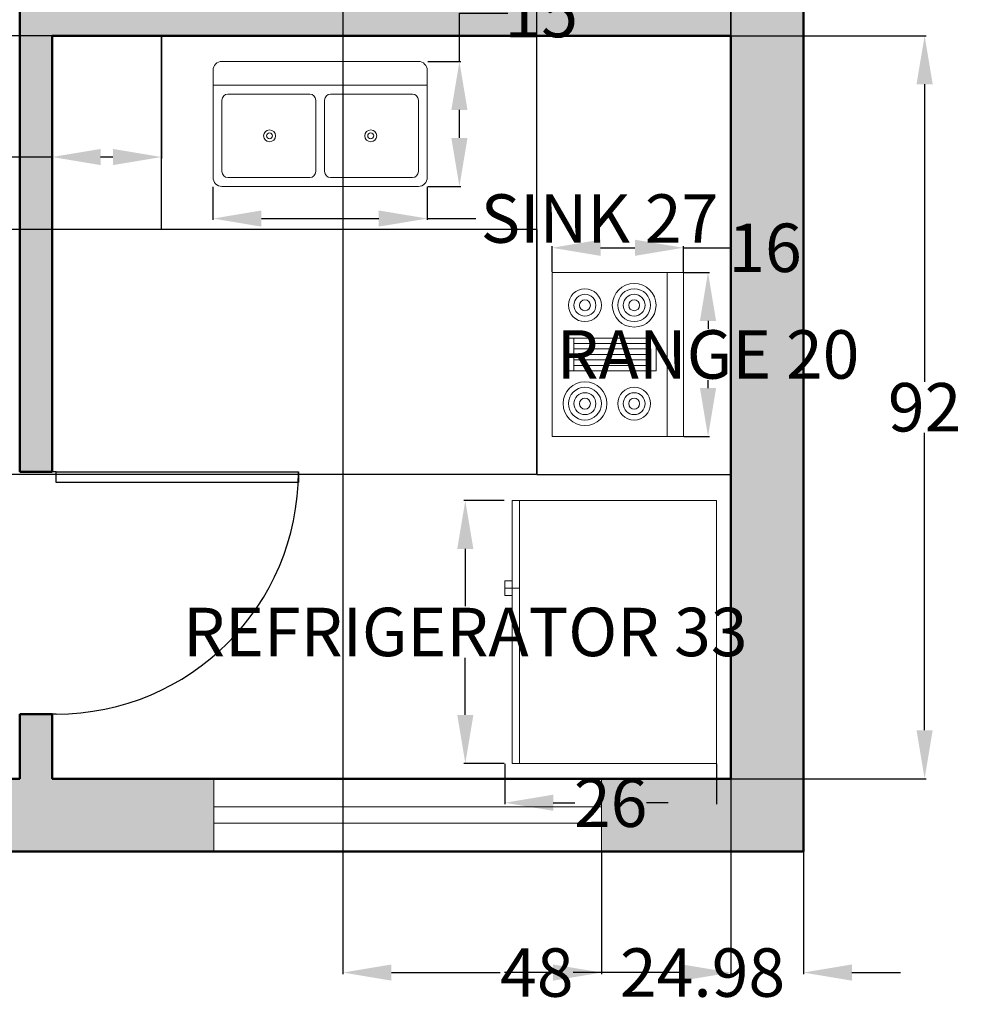
# Model space of a CAD drawing. Units: inches. Extents: x -11 to 341, y -300 to 41.
# Tile 4 of 5: x 192 to 308, y -300 to -178. Entities that reach past the tile are written whole.
import ezdxf

# ---------------------------------------------------------------- set-up
doc = ezdxf.new("R2010")
doc.units = ezdxf.units.IN
doc.header["$MEASUREMENT"] = 0
for name, color, linetype, lineweight in [('A-ANNO-DIMS', 2, 'Continuous', 18), ('A-DOOR', 3, 'Continuous', 25), ('A-EQPM', 8, 'Continuous', 18), ('A-FLOR-CASE', 8, 'Continuous', 25), ('A-FLOR-FIXT', 9, 'Continuous', 18), ('A-GLAZ', 4, 'Continuous', 18), ('A-WALL', 7, 'Continuous', 50), ('A-WALL-PATT', 251, 'Continuous', 13)]:
    doc.layers.add(name, color=color, linetype=linetype, lineweight=lineweight)
doc.styles.get("Standard").update_dxf_attribs({"font": 'arial.ttf'})
doc.dimstyles.get("Standard").update_dxf_attribs({"dimtxt": 6, "dimasz": 6, "dimexe": 0.18, "dimexo": 0.0625, "dimgap": 0.09, "dimtad": 0, "dimtih": 1, "dimtoh": 1, "dimdec": 0, "dimzin": 0, "dimdsep": 46, "dimlunit": 4, "dimtxsty": 'Standard', "dimcen": 0.09, "dimadec": 0, "dimazin": 0, "dimtfac": 1, "dimtdec": 0, "dimtofl": 0, "dimtmove": 0, "dimatfit": 3, "dimfxl": 1, "dimtolj": 1, "dimtzin": 0, "dimarcsym": 0})

# ---------------------------------------------------------------- blocks, each defined once
blk = doc.blocks.new('*U12')
for p, q in [((0, 0), (0, -6)), ((40, 0), (40, -6))]:
    blk.add_line(p, q)
blk.add_lwpolyline([(0, 0), (0, 40), (1.75, 40), (1.75, 0)], close=True)
blk.add_arc((0, 0), 40, 0, 90)
blk = doc.blocks.new('Range-Oven - 30 in top')
for p, q in [((0, -3), (30, -3)), ((12, -6), (18, -6)), ((13, -20), (13, -6)), ((14, -6), (14, -20)), ((15, -20), (15, -6)), ((16, -6), (16, -20)), ((17, -20), (17, -6)), ((18, -20), (12, -20))]:
    blk.add_line(p, q)
for points in [[(0, -24), (0, 0), (30, 0), (30, -24)], [(12, -21), (12, -5), (18, -5), (18, -21)]]:
    blk.add_lwpolyline(points, close=True)
for centre, radius in [((6, -9), 4), ((6, -9), 3), ((6, -9), 2), ((24, -9), 3), ((24, -9), 2), ((6, -9), 1), ((24, -9), 1), ((24, -18), 4), ((6, -18), 3), ((6, -18), 2), ((24, -18), 3), ((24, -18), 2), ((6, -18), 1), ((24, -18), 1)]:
    blk.add_circle(centre, radius)
blk = doc.blocks.new('Sink-double - 36 in top')
for p, q in [((-18, -4), (18, -4)), ((-0.75, -18.5), (-0.75, -6.5)), ((0.75, -6.5), (0.75, -18.5))]:
    blk.add_line(p, q)
for points in [[(-16.5, 0), (16.5, 0)], [(-18, -19.5), (-18, -1.5)], [(18, -1.5), (18, -19.5)], [(-16.5, -18.5), (-16.5, -6.5)], [(-15.5, -5.5), (-1.75, -5.5)], [(1.75, -5.5), (15.5, -5.5)], [(16.5, -6.5), (16.5, -18.5)], [(-1.75, -19.5), (-15.5, -19.5)], [(15.5, -19.5), (1.75, -19.5)], [(16.5, -21), (-16.5, -21)]]:
    blk.add_lwpolyline(points)
for centre, radius in [((-8.5, -12.5), 1), ((8.5, -12.5), 1), ((-8.5, -12.5), 0.5), ((8.5, -12.5), 0.5)]:
    blk.add_circle(centre, radius)
for centre, radius, start, end in [((-16.5, -1.5), 1.5, 90, 180), ((16.5, -1.5), 1.5, 0, 90), ((-15.5, -6.5), 1, 90, 180), ((-1.75, -6.5), 1, 0, 90), ((1.75, -6.5), 1, 90, 180), ((15.5, -6.5), 1, 0, 90), ((-16.5, -19.5), 1.5, 180, 270), ((-15.5, -18.5), 1, 180, 270), ((-1.75, -18.5), 1, 270, 0), ((1.75, -18.5), 1, 180, 270), ((15.5, -18.5), 1, 270, 0), ((16.5, -19.5), 1.5, 270, 0)]:
    blk.add_arc(centre, radius, start, end)
blk = doc.blocks.new('Refrigerator-2 door - 36 in top')
for p, q in [((0, -26.999999), (36, -26.999999)), ((11, -27.999999), (11, -28.999999)), ((12, -26.999999), (12, -28.999999)), ((13, -28.999999), (13, -27.999999)), ((11, -28.999999), (13, -28.999999))]:
    blk.add_line(p, q)
blk.add_lwpolyline([(0, -27.999999), (0, 0), (36, 0), (36, -27.999999)], close=True)
blk = doc.blocks.new('WIN-48IN')
for p, q in [((0, 0), (0, 9)), ((48, 9), (48, 0)), ((0, 5.5), (48, 5.5)), ((0, 3.5), (48, 3.5))]:
    blk.add_line(p, q)
blk = doc.blocks.new('*D35')
at = {"layer": 'A-ANNO-DIMS', "color": 0, "lineweight": -2, "transparency": 16777216}
for p, q in [((273.78, -208.9), (276.94, -208.9)), ((276.76, -214.9), (276.76, -215.87)), ((276.76, -223.22), (276.76, -222.25)), ((273.78, -229.22), (276.94, -229.22))]:
    blk.add_line(p, q, dxfattribs=at)
at = {"layer": 'A-ANNO-DIMS', "color": 0, "transparency": 16777216}
for points in [[(275.76, -214.9), (277.76, -214.9), (276.76, -208.9)], [(275.76, -223.22), (277.76, -223.22), (276.76, -229.22)]]:
    blk.add_solid(points, dxfattribs=at)
at = {"layer": 'Defpoints', "color": 0, "transparency": 16777216}
for p in [(273.72, -208.9), (273.72, -229.22), (276.76, -229.22)]:
    blk.add_point(p, dxfattribs=at)
at = {"layer": 'A-ANNO-DIMS', "color": 0, "transparency": 16777216, "insert": (276.76, -219.06), "char_height": 6, "attachment_point": 5}
blk.add_mtext('\\A1;RANGE 20', dxfattribs=at)
blk = doc.blocks.new('*D36')
at = {"layer": 'A-ANNO-DIMS', "color": 0, "lineweight": -2, "transparency": 16777216}
for p, q in [((257.46, -208.84), (257.46, -205.67)), ((263.46, -205.85), (267.72, -205.85)), ((273.72, -208.84), (273.72, -205.67)), ((273.72, -205.85), (279.72, -205.85))]:
    blk.add_line(p, q, dxfattribs=at)
at = {"layer": 'A-ANNO-DIMS', "color": 0, "transparency": 16777216}
for points in [[(263.46, -204.85), (263.46, -206.85), (257.46, -205.85)], [(267.72, -204.85), (267.72, -206.85), (273.72, -205.85)]]:
    blk.add_solid(points, dxfattribs=at)
at = {"layer": 'Defpoints', "color": 0, "transparency": 16777216}
for p in [(273.72, -205.85), (257.46, -208.9), (273.72, -208.9)]:
    blk.add_point(p, dxfattribs=at)
at = {"layer": 'A-ANNO-DIMS', "color": 0, "transparency": 16777216, "insert": (283.82, -205.85), "char_height": 6, "attachment_point": 5}
blk.add_mtext('\\A1;16', dxfattribs=at)
blk = doc.blocks.new('*D37')
at = {"layer": 'A-ANNO-DIMS', "color": 0, "lineweight": -2, "transparency": 16777216}
for p, q in [((215.49, -198.31), (215.49, -202.41)), ((242.01, -198.31), (242.01, -202.41)), ((221.49, -202.23), (236.01, -202.23)), ((242.01, -202.23), (248.01, -202.23))]:
    blk.add_line(p, q, dxfattribs=at)
at = {"layer": 'A-ANNO-DIMS', "color": 0, "transparency": 16777216}
for points in [[(221.49, -201.23), (221.49, -203.23), (215.49, -202.23)], [(236.01, -201.23), (236.01, -203.23), (242.01, -202.23)]]:
    blk.add_solid(points, dxfattribs=at)
at = {"layer": 'Defpoints', "color": 0, "transparency": 16777216}
for p in [(215.49, -198.25), (242.01, -198.25), (242.01, -202.23)]:
    blk.add_point(p, dxfattribs=at)
at = {"layer": 'A-ANNO-DIMS', "color": 0, "transparency": 16777216, "insert": (263.33, -202.23), "char_height": 6, "attachment_point": 5}
blk.add_mtext('\\A1;SINK 27', dxfattribs=at)
blk = doc.blocks.new('*D38')
at = {"layer": 'A-ANNO-DIMS', "color": 0, "lineweight": -2, "transparency": 16777216}
for p, q in [((245.99, -182.78), (245.99, -176.78)), ((245.99, -176.78), (251.99, -176.78)), ((242.07, -182.78), (246.17, -182.78)), ((245.99, -192.25), (245.99, -188.78)), ((242.07, -198.25), (246.17, -198.25))]:
    blk.add_line(p, q, dxfattribs=at)
at = {"layer": 'A-ANNO-DIMS', "color": 0, "transparency": 16777216}
for points in [[(244.99, -188.78), (246.99, -188.78), (245.99, -182.78)], [(244.99, -192.25), (246.99, -192.25), (245.99, -198.25)]]:
    blk.add_solid(points, dxfattribs=at)
at = {"layer": 'Defpoints', "color": 0, "transparency": 16777216}
for p in [(242.01, -182.78), (245.99, -182.78), (242.01, -198.25)]:
    blk.add_point(p, dxfattribs=at)
at = {"layer": 'A-ANNO-DIMS', "color": 0, "transparency": 16777216, "insert": (256.12, -176.78), "char_height": 6, "attachment_point": 5}
blk.add_mtext('\\A1;15', dxfattribs=at)
blk = doc.blocks.new('*D39')
at = {"layer": 'A-ANNO-DIMS', "color": 0, "lineweight": -2, "transparency": 16777216}
for p, q in [((251.54, -237.15), (246.54, -237.15)), ((246.72, -243.15), (246.72, -250.23)), ((246.72, -263.7), (246.72, -256.62)), ((251.54, -269.7), (246.54, -269.7))]:
    blk.add_line(p, q, dxfattribs=at)
at = {"layer": 'A-ANNO-DIMS', "color": 0, "transparency": 16777216}
for points in [[(245.72, -243.15), (247.72, -243.15), (246.72, -237.15)], [(245.72, -263.7), (247.72, -263.7), (246.72, -269.7)]]:
    blk.add_solid(points, dxfattribs=at)
at = {"layer": 'Defpoints', "color": 0, "transparency": 16777216}
for p in [(251.6, -237.15), (246.72, -269.7), (251.6, -269.7)]:
    blk.add_point(p, dxfattribs=at)
at = {"layer": 'A-ANNO-DIMS', "color": 0, "transparency": 16777216, "insert": (246.72, -253.43), "char_height": 6, "attachment_point": 5}
blk.add_mtext('\\A1;REFRIGERATOR 33', dxfattribs=at)
blk = doc.blocks.new('*D40')
at = {"layer": 'A-ANNO-DIMS', "color": 0, "lineweight": -2, "transparency": 16777216}
for p, q in [((251.6, -269.76), (251.6, -274.76)), ((277.83, -269.76), (277.83, -274.76)), ((257.6, -274.58), (260.28, -274.58)), ((271.83, -274.58), (269.15, -274.58))]:
    blk.add_line(p, q, dxfattribs=at)
at = {"layer": 'A-ANNO-DIMS', "color": 0, "transparency": 16777216}
for points in [[(257.6, -273.58), (257.6, -275.58), (251.6, -274.58)], [(271.83, -273.58), (271.83, -275.58), (277.83, -274.58)]]:
    blk.add_solid(points, dxfattribs=at)
at = {"layer": 'Defpoints', "color": 0, "transparency": 16777216}
for p in [(251.6, -269.7), (277.83, -269.7), (277.83, -274.58)]:
    blk.add_point(p, dxfattribs=at)
at = {"layer": 'A-ANNO-DIMS', "color": 0, "transparency": 16777216, "insert": (264.71, -274.58), "char_height": 6, "attachment_point": 5}
blk.add_mtext('\\A1;26', dxfattribs=at)
blk = doc.blocks.new('*D53')
at = {"layer": 'A-ANNO-DIMS', "color": 0, "lineweight": -2, "transparency": 16777216}
for p, q in [((263.59, -280.67), (263.59, -295.79)), ((288.57, -280.67), (288.57, -295.79)), ((257.59, -295.61), (251.59, -295.61)), ((294.57, -295.61), (300.57, -295.61))]:
    blk.add_line(p, q, dxfattribs=at)
at = {"layer": 'A-ANNO-DIMS', "color": 0, "transparency": 16777216}
for points in [[(257.59, -294.61), (257.59, -296.61), (263.59, -295.61)], [(294.57, -294.61), (294.57, -296.61), (288.57, -295.61)]]:
    blk.add_solid(points, dxfattribs=at)
at = {"layer": 'Defpoints', "color": 0, "transparency": 16777216}
for p in [(263.59, -280.6), (288.57, -280.6), (288.57, -295.61)]:
    blk.add_point(p, dxfattribs=at)
at = {"layer": 'A-ANNO-DIMS', "color": 0, "transparency": 16777216, "insert": (276.08, -295.61), "char_height": 6, "attachment_point": 5}
blk.add_mtext('\\A1;24.98', dxfattribs=at)
blk = doc.blocks.new('*D60')
at = {"layer": 'A-ANNO-DIMS', "color": 0, "lineweight": -2, "transparency": 16777216}
for p, q in [((279.63, -179.6), (303.75, -179.6)), ((303.57, -185.6), (303.57, -222.45)), ((303.57, -265.6), (303.57, -228.76)), ((279.63, -271.6), (303.75, -271.6))]:
    blk.add_line(p, q, dxfattribs=at)
at = {"layer": 'A-ANNO-DIMS', "color": 0, "transparency": 16777216}
for points in [[(302.57, -185.6), (304.57, -185.6), (303.57, -179.6)], [(302.57, -265.6), (304.57, -265.6), (303.57, -271.6)]]:
    blk.add_solid(points, dxfattribs=at)
at = {"layer": 'Defpoints', "color": 0, "transparency": 16777216}
for p in [(279.57, -179.6), (303.57, -179.6), (279.57, -271.6)]:
    blk.add_point(p, dxfattribs=at)
at = {"layer": 'A-ANNO-DIMS', "color": 0, "transparency": 16777216, "insert": (303.57, -225.6), "char_height": 6, "attachment_point": 5}
blk.add_mtext('\\A1;92', dxfattribs=at)
blk = doc.blocks.new('*D63')
at = {"layer": 'A-ANNO-DIMS', "color": 0, "lineweight": -2, "transparency": 16777216}
for p, q in [((231.57, -175.67), (231.57, -295.79)), ((279.57, -175.67), (279.57, -295.79)), ((237.57, -295.61), (251.05, -295.61)), ((273.57, -295.61), (260.08, -295.61))]:
    blk.add_line(p, q, dxfattribs=at)
at = {"layer": 'A-ANNO-DIMS', "color": 0, "transparency": 16777216}
for points in [[(237.57, -294.61), (237.57, -296.61), (231.57, -295.61)], [(273.57, -294.61), (273.57, -296.61), (279.57, -295.61)]]:
    blk.add_solid(points, dxfattribs=at)
at = {"layer": 'Defpoints', "color": 0, "transparency": 16777216}
for p in [(231.57, -175.6), (279.57, -175.6), (279.57, -295.61)]:
    blk.add_point(p, dxfattribs=at)
at = {"layer": 'A-ANNO-DIMS', "color": 0, "transparency": 16777216, "insert": (255.57, -295.61), "char_height": 6, "attachment_point": 5}
blk.add_mtext('\\A1;48', dxfattribs=at)
blk = doc.blocks.new('*D74')
at = {"layer": 'A-ANNO-DIMS', "color": 0, "lineweight": -2, "transparency": 16777216}
for p, q in [((209.05, -179.6), (9.38, -179.6)), ((9.56, -185.6), (9.56, -188.5)), ((9.56, -197.6), (9.56, -194.71)), ((209.05, -203.6), (9.38, -203.6))]:
    blk.add_line(p, q, dxfattribs=at)
at = {"layer": 'A-ANNO-DIMS', "color": 0, "transparency": 16777216}
for points in [[(8.56, -185.6), (10.56, -185.6), (9.56, -179.6)], [(8.56, -197.6), (10.56, -197.6), (9.56, -203.6)]]:
    blk.add_solid(points, dxfattribs=at)
at = {"layer": 'Defpoints', "color": 0, "transparency": 16777216}
for p in [(209.11, -179.6), (9.56, -203.6), (209.11, -203.6)]:
    blk.add_point(p, dxfattribs=at)
at = {"layer": 'A-ANNO-DIMS', "color": 0, "transparency": 16777216, "insert": (9.56, -191.6), "char_height": 6, "attachment_point": 5}
blk.add_mtext('\\A1;24', dxfattribs=at)
blk = doc.blocks.new('*D75')
at = {"layer": 'A-ANNO-DIMS', "color": 0, "lineweight": -2, "transparency": 16777216}
for p, q in [((195.57, -179.67), (195.57, -194.79)), ((209.11, -179.67), (209.11, -194.79)), ((195.57, -194.61), (189.57, -194.61)), ((203.11, -194.61), (201.57, -194.61))]:
    blk.add_line(p, q, dxfattribs=at)
at = {"layer": 'A-ANNO-DIMS', "color": 0, "transparency": 16777216}
for points in [[(201.57, -193.61), (201.57, -195.61), (195.57, -194.61)], [(203.11, -193.61), (203.11, -195.61), (209.11, -194.61)]]:
    blk.add_solid(points, dxfattribs=at)
at = {"layer": 'Defpoints', "color": 0, "transparency": 16777216}
for p in [(195.57, -179.6), (209.11, -179.6), (195.57, -194.61)]:
    blk.add_point(p, dxfattribs=at)
at = {"layer": 'A-ANNO-DIMS', "color": 0, "transparency": 16777216, "insert": (179.61, -194.61), "char_height": 6, "attachment_point": 5}
blk.add_mtext('\\A1;13.55', dxfattribs=at)
blk = doc.blocks.new('*D76')
at = {"layer": 'A-ANNO-DIMS', "color": 0, "lineweight": -2, "transparency": 16777216}
for p, q in [((255.5, -203.6), (9.38, -203.6)), ((9.56, -209.6), (9.56, -215.6)), ((9.56, -227.91), (9.56, -221.91)), ((255.5, -233.91), (9.38, -233.91))]:
    blk.add_line(p, q, dxfattribs=at)
at = {"layer": 'A-ANNO-DIMS', "color": 0, "transparency": 16777216}
for points in [[(8.56, -209.6), (10.56, -209.6), (9.56, -203.6)], [(8.56, -227.91), (10.56, -227.91), (9.56, -233.91)]]:
    blk.add_solid(points, dxfattribs=at)
at = {"layer": 'Defpoints', "color": 0, "transparency": 16777216}
for p in [(9.56, -203.6), (255.57, -203.6), (255.57, -233.91)]:
    blk.add_point(p, dxfattribs=at)
at = {"layer": 'A-ANNO-DIMS', "color": 0, "transparency": 16777216, "insert": (9.56, -218.76), "char_height": 6, "attachment_point": 5}
blk.add_mtext('\\A1;30.307', dxfattribs=at)
blk = doc.blocks.new('*D77')
at = {"layer": 'A-ANNO-DIMS', "color": 0, "lineweight": -2, "transparency": 16777216}
for p, q in [((255.57, -233.85), (255.57, 34.58)), ((261.57, 34.4), (263.14, 34.4)), ((273.57, 34.4), (271.99, 34.4)), ((279.57, -233.85), (279.57, 34.58))]:
    blk.add_line(p, q, dxfattribs=at)
at = {"layer": 'A-ANNO-DIMS', "color": 0, "transparency": 16777216}
for points in [[(261.57, 35.4), (261.57, 33.4), (255.57, 34.4)], [(273.57, 35.4), (273.57, 33.4), (279.57, 34.4)]]:
    blk.add_solid(points, dxfattribs=at)
at = {"layer": 'Defpoints', "color": 0, "transparency": 16777216}
for p in [(279.57, 34.4), (255.57, -233.91), (279.57, -233.91)]:
    blk.add_point(p, dxfattribs=at)
at = {"layer": 'A-ANNO-DIMS', "color": 0, "transparency": 16777216, "insert": (267.57, 34.4), "char_height": 6, "attachment_point": 5}
blk.add_mtext('\\A1;24', dxfattribs=at)

msp = doc.modelspace()

# ---------------------------------------------------------------- hatches: boundary and pattern name
at = {"layer": 'A-WALL-PATT'}
h = msp.add_hatch(color=256, dxfattribs=at)
h.dxf.hatch_style = 1
h.paths.add_polyline_path([(231.5651, -175.6033), (231.5651, -127.6033), (227.5651, -127.6033), (227.5651, -175.6033), (191.5651, -175.6033), (191.5651, -233.6033), (195.5651, -233.6033), (195.5651, -179.6033), (279.5651, -179.6033), (279.5651, -271.6033), (263.5868, -271.6033), (263.5868, -280.6033), (288.5651, -280.6033), (288.5651, -132.6033), (279.5651, -132.6033), (279.5651, -175.6033)])
h = msp.add_hatch(color=256, dxfattribs=at)
h.dxf.hatch_style = 1
h.paths.add_polyline_path([(215.5868, -280.6033), (215.5868, -271.6033), (195.5651, -271.6033), (195.5651, -263.6033), (191.5651, -263.6033), (191.5651, -271.6033), (165.5651, -271.6033), (165.5651, -280.6033)])

# ---------------------------------------------------------------- linework, layer by layer
at = {"layer": 'A-FLOR-CASE'}
for p, q in [((209.1143, -203.6033), (209.1143, -179.6033)), ((255.5651, -203.6033), (209.1143, -203.6033)), ((255.5651, -203.6033), (255.5651, -233.9102)), ((255.5651, -233.9102), (279.5651, -233.9102))]:
    msp.add_line(p, q, dxfattribs=at)
at = {"layer": 'A-WALL'}
for p, q in [((191.5651, -175.6033), (191.5651, -233.6033)), ((279.5651, -179.6033), (195.5651, -179.6033)), ((195.5651, -179.6033), (195.5651, -233.6033)), ((279.5651, -179.6033), (279.5651, -271.6033)), ((191.5651, -233.6033), (195.5651, -233.6033)), ((191.5651, -263.6033), (195.5651, -263.6033)), ((191.5651, -263.6033), (191.5651, -271.6033)), ((195.5651, -263.6033), (195.5651, -271.6033)), ((191.5651, -271.6033), (165.5651, -271.6033)), ((279.5651, -271.6033), (195.5651, -271.6033))]:
    msp.add_line(p, q, dxfattribs=at)
msp.add_lwpolyline([(129.5651, -280.6033), (24.5651, -280.6033), (24.5651, 19.3967), (288.5651, 19.3967), (288.5651, -280.6033), (165.5651, -280.6033)], dxfattribs=at)

# ---------------------------------------------------------------- block references
at = {"layer": 'A-DOOR', "xscale": 0.75, "yscale": 0.75, "zscale": 0.75, "rotation": 270}
msp.add_blockref('*U12', (196.0651, -233.6033), dxfattribs=at)
at = {"layer": 'A-EQPM', "rotation": 270}
for name, p, xscale, yscale, zscale in [('Range-Oven - 30 in top', (273.7163, -208.9012), 0.677253776970797, 0.677253776970797, 0.677253776970797), ('Refrigerator-2 door - 36 in top', (277.8255, -237.1503), 0.9041759814694595, 0.9041759814694595, 0.9041759814694595)]:
    msp.add_blockref(name, p, dxfattribs=dict(at, xscale=xscale, yscale=yscale, zscale=zscale))
at = {"layer": 'A-FLOR-FIXT', "xscale": 0.7366845539354328, "yscale": 0.7366845539354328, "zscale": 0.7366845539354328}
msp.add_blockref('Sink-double - 36 in top', (228.752, -182.7778), dxfattribs=at)
at = {"layer": 'A-GLAZ'}
msp.add_blockref('WIN-48IN', (215.5868, -280.603), dxfattribs=at)

# ---------------------------------------------------------------- dimensions: what is measured, and where the dimension line sits
at = {"layer": 'A-ANNO-DIMS'}
for base, p1, p2, override, picture, middle in [((279.5651, 34.3987), (255.5651, -233.9102), (279.5651, -233.9102), {"dimdec": 0, "dimlfac": 1, "dimrnd": 0, "dimzin": 0, "dimdsep": 46, "dimlunit": 2}, '*D77', (267.5651, 34.3987)), ((279.5651, -295.6053), (231.5651, -175.6033), (279.5651, -175.6033), {"dimdec": 0, "dimlfac": 1, "dimrnd": 0, "dimzin": 0, "dimdsep": 46, "dimlunit": 2}, '*D63', (255.5651, -295.6053)), ((273.7163, -205.8536), (257.4623, -208.9012), (273.7163, -208.9012), {"dimdec": 0, "dimlfac": 1, "dimrnd": 0, "dimzin": 0, "dimdsep": 46, "dimlunit": 2}, '*D36', (283.8193, -205.8536)), ((277.8255, -274.5832), (251.6044, -269.7006), (277.8255, -269.7006), {"dimdec": 0, "dimlfac": 1, "dimrnd": 0, "dimzin": 0, "dimdsep": 46, "dimlunit": 2}, '*D40', (264.7149, -274.5832)), ((288.5651, -295.6053), (263.5868, -280.6033), (288.5651, -280.6033), {"dimdec": 2, "dimlfac": 1, "dimrnd": 0, "dimzin": 0, "dimdsep": 46, "dimlunit": 2}, '*D53', (276.076, -295.6053))]:
    dim = msp.add_linear_dim(base=base, p1=p1, p2=p2, dimstyle='Standard', override=override, dxfattribs=at)
    dim.commit()
    dim.dimension.update_dxf_attribs({"geometry": picture, "text_midpoint": middle})
for base, p1, p2, angle, override, picture, middle in [((245.9904, -182.7778), (242.0123, -198.2482), (242.0123, -182.7778), 90, {"dimdec": 0, "dimlfac": 1, "dimrnd": 0, "dimzin": 0, "dimdsep": 46, "dimlunit": 2}, '*D38', (256.1179, -176.7778)), ((9.5631, -203.6033), (209.1143, -179.6033), (209.1143, -203.6033), 90, {"dimdec": 0, "dimlfac": 1, "dimrnd": 0, "dimzin": 0, "dimdsep": 46, "dimlunit": 2}, '*D74', (9.5631, -191.6033)), ((195.5651, -194.6053), (209.1143, -179.6033), (195.5651, -179.6033), 180, {"dimdec": 2, "dimlfac": 1, "dimrnd": 0, "dimzin": 0, "dimdsep": 46, "dimlunit": 2}, '*D75', (179.6115, -194.6053)), ((303.5671, -179.6033), (279.5651, -271.6033), (279.5651, -179.6033), 90, {"dimdec": 0, "dimlfac": 1, "dimrnd": 0, "dimzin": 0, "dimdsep": 46, "dimlunit": 2}, '*D60', (303.5671, -225.6033)), ((9.5631, -203.6033), (255.5651, -233.9102), (255.5651, -203.6033), 90, {"dimdec": 3, "dimlfac": 1, "dimrnd": 0, "dimzin": 0, "dimdsep": 46, "dimlunit": 2}, '*D76', (9.5631, -218.7567))]:
    dim = msp.add_linear_dim(base=base, p1=p1, p2=p2, angle=angle, dimstyle='Standard', override=override, dxfattribs=at)
    dim.commit()
    dim.dimension.update_dxf_attribs({"geometry": picture, "text_midpoint": middle})
dim = msp.add_linear_dim(base=(242.0123, -202.2263), p1=(215.4917, -198.2482), p2=(242.0123, -198.2482), text='SINK <>', dimstyle='Standard', override={"dimdec": 0, "dimlfac": 1, "dimrnd": 0, "dimzin": 0, "dimdsep": 46, "dimlunit": 2}, dxfattribs=at)
dim.commit()
dim.dimension.update_dxf_attribs({"geometry": '*D37', "text_midpoint": (263.3315, -202.2263)})
for base, p1, p2, text, picture, middle in [((276.764, -229.2189), (273.7163, -208.9012), (273.7163, -229.2189), 'RANGE <>', '*D35', (276.764, -219.0601)), ((246.7218, -269.7006), (251.6044, -237.1503), (251.6044, -269.7006), 'REFRIGERATOR <>', '*D39', (246.7218, -253.4255))]:
    dim = msp.add_linear_dim(base=base, p1=p1, p2=p2, angle=270, text=text, dimstyle='Standard', override={"dimdec": 0, "dimlfac": 1, "dimrnd": 0, "dimzin": 0, "dimdsep": 46, "dimlunit": 2}, dxfattribs=at)
    dim.commit()
    dim.dimension.update_dxf_attribs({"geometry": picture, "text_midpoint": middle})

doc.saveas('drawing.dxf')
